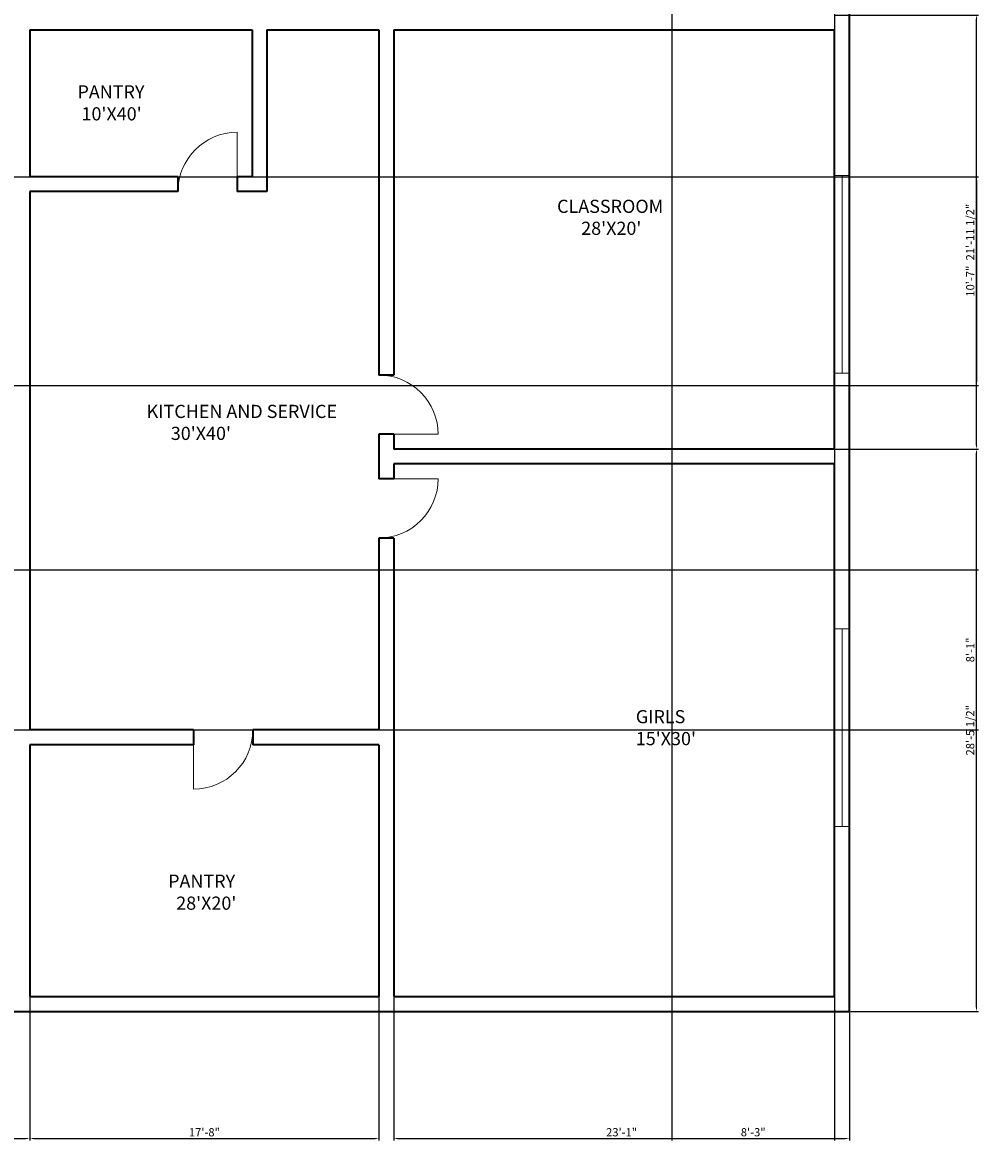
# Model space of a CAD drawing. Units: inches. Extents: x 2394 to 4066, y 1878 to 3193.
# Tile 2 of 3: x 3482 to 4066, y 1878 to 2560. Entities that reach past the tile are written whole.
import ezdxf

# ---------------------------------------------------------------- set-up
doc = ezdxf.new("R2010")
doc.units = ezdxf.units.IN
for name, color, linetype, lineweight in [('A-ANNO-DIMS', 2, 'Continuous', 13), ('A-AREA-IDEN', 7, 'Continuous', 18), ('A-DOOR', 3, 'Continuous', 18), ('A-GLAZ', 4, 'Continuous', 18), ('A-WALL', 7, 'Continuous', 35)]:
    doc.layers.add(name, color=color, linetype=linetype, lineweight=lineweight)
doc.styles.get("Standard").update_dxf_attribs({"font": 'arial.ttf'})
doc.dimstyles.new('ISO-25', dxfattribs={"dimtxt": 5, "dimasz": 2.5, "dimexe": 1.25, "dimexo": 0.625, "dimtad": 1, "dimlunit": 3, "dimtxsty": 'Standard', "dimcen": 2.5, "dimadec": 0, "dimazin": 0, "dimtfac": 1, "dimtmove": 0, "dimatfit": 3, "dimfxl": 1, "dimarcsym": 0})

# ---------------------------------------------------------------- blocks, each defined once
blk = doc.blocks.new('DOOR-SINGLE-36IN')
blk.add_line((36, 0), (36, 36))
blk.add_arc((36, 0), 36, 90, 180)
blk = doc.blocks.new('WINDOW-120IN')
for p, q in [((0, 0), (0, 9)), ((120, 0), (120, 9)), ((120, 4.5), (0, 4.5))]:
    blk.add_line(p, q)
blk = doc.blocks.new('*D23')
at = {"layer": 'A-ANNO-DIMS', "color": 0, "lineweight": -2, "transparency": 16777216}
for p, q in [((2986.6, 1967.47), (2986.6, 1880.59)), ((3486.1, 1967.47), (3486.1, 1880.59)), ((2989.1, 1881.84), (3483.6, 1881.84))]:
    blk.add_line(p, q, dxfattribs=at)
at = {"layer": 'A-ANNO-DIMS', "color": 0, "transparency": 16777216}
for points in [[(2989.1, 1882.26), (2989.1, 1881.43), (2986.6, 1881.84)], [(3483.6, 1882.26), (3483.6, 1881.43), (3486.1, 1881.84)]]:
    blk.add_solid(points, dxfattribs=at)
at = {"layer": 'Defpoints', "color": 0, "transparency": 16777216}
for p in [(2986.6, 1968.09), (3486.1, 1968.09), (3486.1, 1881.84)]:
    blk.add_point(p, dxfattribs=at)
at = {"layer": 'A-ANNO-DIMS', "color": 0, "transparency": 16777216, "insert": (3236.35, 1885.05), "char_height": 5, "attachment_point": 5}
blk.add_mtext('41\'-7 1/2"', dxfattribs=at)
blk = doc.blocks.new('*D24')
at = {"layer": 'A-ANNO-DIMS', "color": 0, "lineweight": -2, "transparency": 16777216}
for p, q in [((3486.1, 2120.47), (3486.1, 1880.59)), ((3698.2, 2120.47), (3698.2, 1880.59)), ((3488.6, 1881.84), (3695.7, 1881.84))]:
    blk.add_line(p, q, dxfattribs=at)
at = {"layer": 'A-ANNO-DIMS', "color": 0, "transparency": 16777216}
for points in [[(3488.6, 1882.26), (3488.6, 1881.43), (3486.1, 1881.84)], [(3695.7, 1882.26), (3695.7, 1881.43), (3698.2, 1881.84)]]:
    blk.add_solid(points, dxfattribs=at)
at = {"layer": 'Defpoints', "color": 0, "transparency": 16777216}
for p in [(3486.1, 2121.09), (3698.2, 2121.09), (3698.2, 1881.84)]:
    blk.add_point(p, dxfattribs=at)
at = {"layer": 'A-ANNO-DIMS', "color": 0, "transparency": 16777216, "insert": (3592.15, 1885.02), "char_height": 5, "attachment_point": 5}
blk.add_mtext('17\'-8"', dxfattribs=at)
blk = doc.blocks.new('*D25')
at = {"layer": 'A-ANNO-DIMS', "color": 0, "lineweight": -2, "transparency": 16777216}
for p, q in [((3707.2, 1967.47), (3707.2, 1880.59)), ((3984.1, 1958.47), (3984.1, 1880.59)), ((3709.7, 1881.84), (3981.6, 1881.84))]:
    blk.add_line(p, q, dxfattribs=at)
at = {"layer": 'A-ANNO-DIMS', "color": 0, "transparency": 16777216}
for points in [[(3709.7, 1882.26), (3709.7, 1881.43), (3707.2, 1881.84)], [(3981.6, 1882.26), (3981.6, 1881.43), (3984.1, 1881.84)]]:
    blk.add_solid(points, dxfattribs=at)
at = {"layer": 'Defpoints', "color": 0, "transparency": 16777216}
for p in [(3707.2, 1968.09), (3984.1, 1959.09), (3984.1, 1881.84)]:
    blk.add_point(p, dxfattribs=at)
at = {"layer": 'A-ANNO-DIMS', "color": 0, "transparency": 16777216, "insert": (3845.65, 1885.02), "char_height": 5, "attachment_point": 5}
blk.add_mtext('23\'-1"', dxfattribs=at)
blk = doc.blocks.new('*D26')
at = {"layer": 'A-ANNO-DIMS', "color": 0, "lineweight": -2, "transparency": 16777216}
for p, q in [((3975.72, 2300.64), (4062.6, 2300.64)), ((4061.35, 1961.59), (4061.35, 2298.14)), ((3984.72, 1959.09), (4062.6, 1959.09))]:
    blk.add_line(p, q, dxfattribs=at)
at = {"layer": 'A-ANNO-DIMS', "color": 0, "transparency": 16777216}
for points in [[(4060.93, 2298.14), (4061.76, 2298.14), (4061.35, 2300.64)], [(4060.93, 1961.59), (4061.76, 1961.59), (4061.35, 1959.09)]]:
    blk.add_solid(points, dxfattribs=at)
at = {"layer": 'Defpoints', "color": 0, "transparency": 16777216}
for p in [(3975.1, 2300.64), (4061.35, 2300.64), (3984.1, 1959.09)]:
    blk.add_point(p, dxfattribs=at)
at = {"layer": 'A-ANNO-DIMS', "color": 0, "transparency": 16777216, "insert": (4058.14, 2129.87), "char_height": 5, "attachment_point": 5, "rotation": 90}
blk.add_mtext('28\'-5 1/2"', dxfattribs=at)
blk = doc.blocks.new('*D27')
at = {"layer": 'A-ANNO-DIMS', "color": 0, "lineweight": -2, "transparency": 16777216}
for p, q in [((3975.72, 2564.33), (4062.6, 2564.33)), ((4061.35, 2303.14), (4061.35, 2561.83)), ((3975.72, 2300.64), (4062.6, 2300.64))]:
    blk.add_line(p, q, dxfattribs=at)
at = {"layer": 'A-ANNO-DIMS', "color": 0, "transparency": 16777216}
for points in [[(4060.93, 2561.83), (4061.76, 2561.83), (4061.35, 2564.33)], [(4060.93, 2303.14), (4061.76, 2303.14), (4061.35, 2300.64)]]:
    blk.add_solid(points, dxfattribs=at)
at = {"layer": 'Defpoints', "color": 0, "transparency": 16777216}
for p in [(3975.1, 2564.33), (4061.35, 2564.33), (3975.1, 2300.64)]:
    blk.add_point(p, dxfattribs=at)
at = {"layer": 'A-ANNO-DIMS', "color": 0, "transparency": 16777216, "insert": (4058.14, 2432.49), "char_height": 5, "attachment_point": 5, "rotation": 90}
blk.add_mtext('21\'-11 1/2"', dxfattribs=at)
blk = doc.blocks.new('*D29')
at = {"layer": 'A-ANNO-DIMS', "color": 0, "lineweight": -2, "transparency": 16777216}
for p, q in [((2814.72, 2466.09), (4062.6, 2466.09)), ((4061.35, 2463.59), (4061.35, 2341.75)), ((2814.72, 2339.25), (4062.6, 2339.25))]:
    blk.add_line(p, q, dxfattribs=at)
at = {"layer": 'A-ANNO-DIMS', "color": 0, "transparency": 16777216}
for points in [[(4060.93, 2463.59), (4061.76, 2463.59), (4061.35, 2466.09)], [(4060.93, 2341.75), (4061.76, 2341.75), (4061.35, 2339.25)]]:
    blk.add_solid(points, dxfattribs=at)
at = {"layer": 'Defpoints', "color": 0, "transparency": 16777216}
for p in [(2814.1, 2466.09), (2814.1, 2339.25), (4061.35, 2339.25)]:
    blk.add_point(p, dxfattribs=at)
at = {"layer": 'A-ANNO-DIMS', "color": 0, "transparency": 16777216, "insert": (4058.17, 2402.67), "char_height": 5, "attachment_point": 5, "rotation": 90}
blk.add_mtext('10\'-7"', dxfattribs=at)
blk = doc.blocks.new('*D33')
at = {"layer": 'A-ANNO-DIMS', "color": 0, "lineweight": -2, "transparency": 16777216}
for p, q in [((3876.16, 3095.47), (3876.16, 1880.59)), ((3975.1, 3095.47), (3975.1, 1880.59)), ((3878.66, 1881.84), (3972.6, 1881.84))]:
    blk.add_line(p, q, dxfattribs=at)
at = {"layer": 'A-ANNO-DIMS', "color": 0, "transparency": 16777216}
for points in [[(3878.66, 1882.26), (3878.66, 1881.43), (3876.16, 1881.84)], [(3972.6, 1882.26), (3972.6, 1881.43), (3975.1, 1881.84)]]:
    blk.add_solid(points, dxfattribs=at)
at = {"layer": 'Defpoints', "color": 0, "transparency": 16777216}
for p in [(3876.16, 3096.09), (3975.1, 3096.09), (3975.1, 1881.84)]:
    blk.add_point(p, dxfattribs=at)
at = {"layer": 'A-ANNO-DIMS', "color": 0, "transparency": 16777216, "insert": (3925.63, 1885.02), "char_height": 5, "attachment_point": 5}
blk.add_mtext('8\'-3"', dxfattribs=at)
blk = doc.blocks.new('*D34')
at = {"layer": 'A-ANNO-DIMS', "color": 0, "lineweight": -2, "transparency": 16777216}
for p, q in [((2487.72, 2227.22), (4062.6, 2227.22)), ((4061.35, 2132.59), (4061.35, 2224.72)), ((2487.72, 2130.09), (4062.6, 2130.09))]:
    blk.add_line(p, q, dxfattribs=at)
at = {"layer": 'A-ANNO-DIMS', "color": 0, "transparency": 16777216}
for points in [[(4060.93, 2224.72), (4061.76, 2224.72), (4061.35, 2227.22)], [(4060.93, 2132.59), (4061.76, 2132.59), (4061.35, 2130.09)]]:
    blk.add_solid(points, dxfattribs=at)
at = {"layer": 'Defpoints', "color": 0, "transparency": 16777216}
for p in [(2487.1, 2227.22), (4061.35, 2227.22), (2487.1, 2130.09)]:
    blk.add_point(p, dxfattribs=at)
at = {"layer": 'A-ANNO-DIMS', "color": 0, "transparency": 16777216, "insert": (4058.17, 2178.66), "char_height": 5, "attachment_point": 5, "rotation": 90}
blk.add_mtext('8\'-1"', dxfattribs=at)

msp = doc.modelspace()

# ---------------------------------------------------------------- linework, layer by layer
at = {"layer": 'A-WALL'}
for p, q in [((3984.098, 1959.092), (3984.098, 3105.092)), ((3486.098, 2555.327), (3486.098, 2466.092)), ((3486.098, 2555.327), (3621.098, 2555.327)), ((3621.098, 2555.327), (3621.098, 2466.092)), ((3630.098, 2555.327), (3630.098, 2457.092)), ((3630.098, 2555.327), (3698.204, 2555.327)), ((3698.204, 2555.327), (3698.204, 2345.645)), ((3707.204, 2555.327), (3975.098, 2555.327)), ((3707.204, 2555.327), (3707.204, 2345.645)), ((3975.098, 2300.645), (3975.098, 2555.327)), ((3576.098, 2466.092), (3486.098, 2466.092)), ((3576.098, 2466.092), (3576.098, 2457.092)), ((3621.098, 2466.092), (3612.098, 2466.092)), ((3612.098, 2466.092), (3612.098, 2457.092)), ((3707.204, 2466.092), (3707.204, 2466.092)), ((3576.098, 2457.092), (3486.098, 2457.092)), ((3486.098, 2457.092), (3486.098, 2130.092)), ((3630.098, 2457.092), (3612.098, 2457.092)), ((3707.204, 2457.092), (3707.204, 2345.645)), ((3975.098, 2300.645), (3975.098, 2457.092)), ((3707.204, 2345.645), (3698.204, 2345.645)), ((3707.204, 2309.645), (3698.204, 2309.645)), ((3698.204, 2309.645), (3698.204, 2282.645)), ((3707.204, 2309.645), (3707.204, 2300.645)), ((3975.098, 2300.645), (3707.204, 2300.645)), ((3975.098, 2291.645), (3707.204, 2291.645)), ((3707.204, 2291.645), (3707.204, 2282.645)), ((3975.098, 1968.092), (3975.098, 2291.645)), ((3707.204, 2282.645), (3698.204, 2282.645)), ((3707.204, 2246.645), (3698.204, 2246.645)), ((3698.204, 2246.645), (3698.204, 2130.092)), ((3707.204, 2246.645), (3707.204, 1968.092)), ((3585.594, 2130.092), (3486.098, 2130.092)), ((3585.594, 2130.092), (3585.594, 2121.092)), ((3621.594, 2130.092), (3621.594, 2121.092)), ((3698.204, 2130.092), (3621.594, 2130.092)), ((3486.098, 2121.092), (3486.098, 1968.092)), ((3585.594, 2121.092), (3486.098, 2121.092)), ((3698.204, 2121.092), (3621.594, 2121.092)), ((3698.204, 2121.092), (3698.204, 1968.092)), ((3486.098, 1968.092), (3698.204, 1968.092)), ((3707.204, 1968.092), (3975.098, 1968.092)), ((2478.098, 1959.092), (3984.098, 1959.092))]:
    msp.add_line(p, q, dxfattribs=at)

# ---------------------------------------------------------------- block references
at = {"layer": 'A-DOOR'}
msp.add_blockref('DOOR-SINGLE-36IN', (3576.098, 2457.092), dxfattribs=at)
for p, rotation in [((3698.204, 2345.644), 270.0000000000003), ((3621.594, 2130.092), 180)]:
    msp.add_blockref('DOOR-SINGLE-36IN', p, dxfattribs=dict(at, rotation=rotation))
at = {"layer": 'A-DOOR', "extrusion": (0, 0, -1), "zscale": -1, "rotation": 89.99999999999999}
msp.add_blockref('DOOR-SINGLE-36IN', (-3698.204, 2246.645), dxfattribs=at)
at = {"layer": 'A-GLAZ', "rotation": 90.00000000000006}
for p in [(3984.098, 2346.861), (3984.098, 2071.389)]:
    msp.add_blockref('WINDOW-120IN', p, dxfattribs=at)

# ---------------------------------------------------------------- texts
at = {"layer": 'A-AREA-IDEN', "char_height": 8, "attachment_point": 1}
for s, insert in [("PANTRY\\P 10'X40'", (3515.035, 2521.668)), ("CLASSROOM\\P      28'X20'", (3806.453, 2452.134)), ("KITCHEN AND SERVICE\\P      30'X40'", (3557.08, 2327.551)), ("GIRLS\\P15'X30'", (3854.298, 2142.127)), ("PANTRY\\P  28'X20'", (3570.129, 2042.171))]:
    msp.add_mtext_dynamic_manual_height_columns(s, width=162.41234, gutter_width=12.5, heights=[0], dxfattribs=dict(at, insert=insert))

# ---------------------------------------------------------------- dimensions: what is measured, and where the dimension line sits
at = {"layer": 'A-ANNO-DIMS'}
for base, p1, p2, picture, middle in [((3975.098, 1881.842), (3876.157, 3096.092), (3975.098, 3096.092), '*D33', (3925.627, 1885.022)), ((3698.204, 1881.842), (3486.098, 2121.092), (3698.204, 2121.092), '*D24', (3592.151, 1885.02)), ((3486.098, 1881.842), (2986.598, 1968.092), (3486.098, 1968.092), '*D23', (3236.348, 1885.052)), ((3984.098, 1881.842), (3707.204, 1968.092), (3984.098, 1959.092), '*D25', (3845.651, 1885.022))]:
    dim = msp.add_linear_dim(base=base, p1=p1, p2=p2, dimstyle='ISO-25', override={"dimdec": 1, "dimlfac": 1, "dimrnd": 0, "dimzin": 1, "dimdsep": 46, "dimlunit": 4, "dimfrac": 2}, dxfattribs=at)
    dim.commit()
    dim.dimension.update_dxf_attribs({"geometry": picture, "text_midpoint": middle})
for base, p1, p2, picture, middle in [((4061.348, 2564.327), (3975.098, 2300.645), (3975.098, 2564.327), '*D27', (4058.137, 2432.486)), ((4061.348, 2339.252), (2814.098, 2466.092), (2814.098, 2339.252), '*D29', (4058.17, 2402.672)), ((4061.348, 2300.645), (3984.098, 1959.092), (3975.098, 2300.645), '*D26', (4058.137, 2129.868)), ((4061.348, 2227.22), (2487.098, 2130.092), (2487.098, 2227.22), '*D34', (4058.17, 2178.656))]:
    dim = msp.add_linear_dim(base=base, p1=p1, p2=p2, angle=90, dimstyle='ISO-25', override={"dimdec": 1, "dimlfac": 1, "dimrnd": 0, "dimzin": 1, "dimdsep": 46, "dimlunit": 4, "dimfrac": 2}, dxfattribs=at)
    dim.commit()
    dim.dimension.update_dxf_attribs({"geometry": picture, "text_midpoint": middle})

doc.saveas('drawing.dxf')
